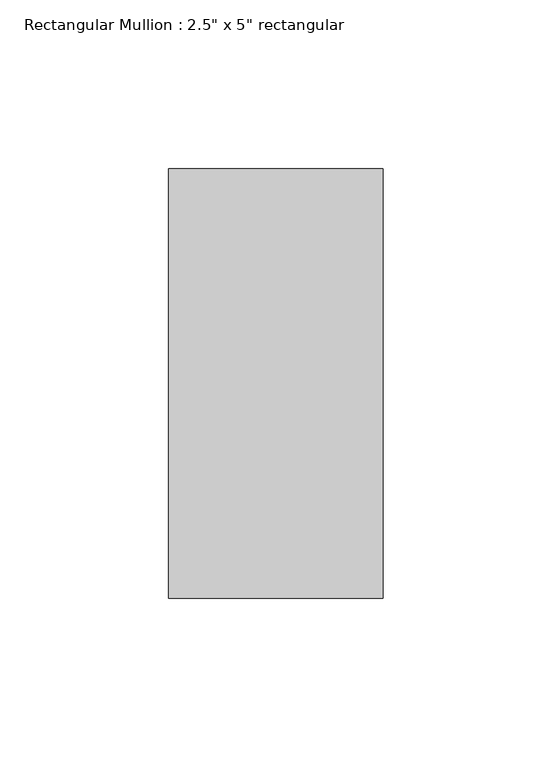
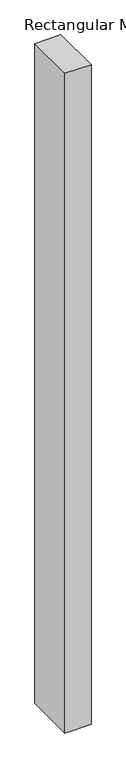
"""IFC4 building model written with IfcOpenShell, lengths in millimetres: member geometry."""

from ifc_helpers import new_model, si_unit, frame, origin, place, context, project, spatial, polyline, outline, extrude, source, transform, mapped, element, save


def member_07726a47(model_context):
    return source(origin(), model_context, "Body", "SweptSolid", [
        extrude(outline(polyline([(31.75, 63.5), (31.75, -63.5), (-31.75, -63.5), (-31.75, 63.5), (31.75, 63.5)])), frame((0.0, 0.0, -1700.4017583), z_axis=(0.0, 0.0, 1.0), x_axis=(1.0, 0.0, 0.0)), (0.0, 0.0, 1.0), 1700.4017583),
    ])


if __name__ == "__main__":
    model = new_model("IFC4")
    model_context = context("Model", 3, world=origin())
    ifc_project = project(units=[si_unit("LENGTHUNIT", "METRE", prefix="MILLI")], contexts=[model_context])
    site = spatial("IfcSite", under=ifc_project)
    building = spatial("IfcBuilding", under=site)
    placement = place(None, origin())
    member_shape = member_07726a47(model_context)
    element("IfcMember", 1, ObjectType="Rectangular Mullion : 2.5\" x 5\" rectangular", at=placement, inside=building, context=model_context, shape_type="MappedRepresentation", body=[
        mapped(member_shape, transform((0.0, 0.0, 0.0), x_axis=(1.0, 0.0, 0.0), y_axis=(0.0, 1.0, 0.0), z_axis=(0.0, 0.0, 1.0))),
    ])
    save(model, "model.ifc")

# Revit data of these elements
# Type "Rectangular Mullion : 2.5\" x 5\" rectangular"
#   built-in parameter 1007304 = 0.416667 (stored number, unit not read)
#   built-in parameter 1007301 = 0.104167 (stored number, unit not read)
#   built-in parameter 1007300 = 0.104167 (stored number, unit not read)
# Element 1 (IfcMember, "Rectangular Mullion : 2.5\" x 5\" rectangular")
#   Materials on its faces: "Aluminum"
# Materials
#   "Aluminum": class "Metal", colour RGB 247 247 247, transparency 0, Description = "Aluminum 6061", Cost = 0
